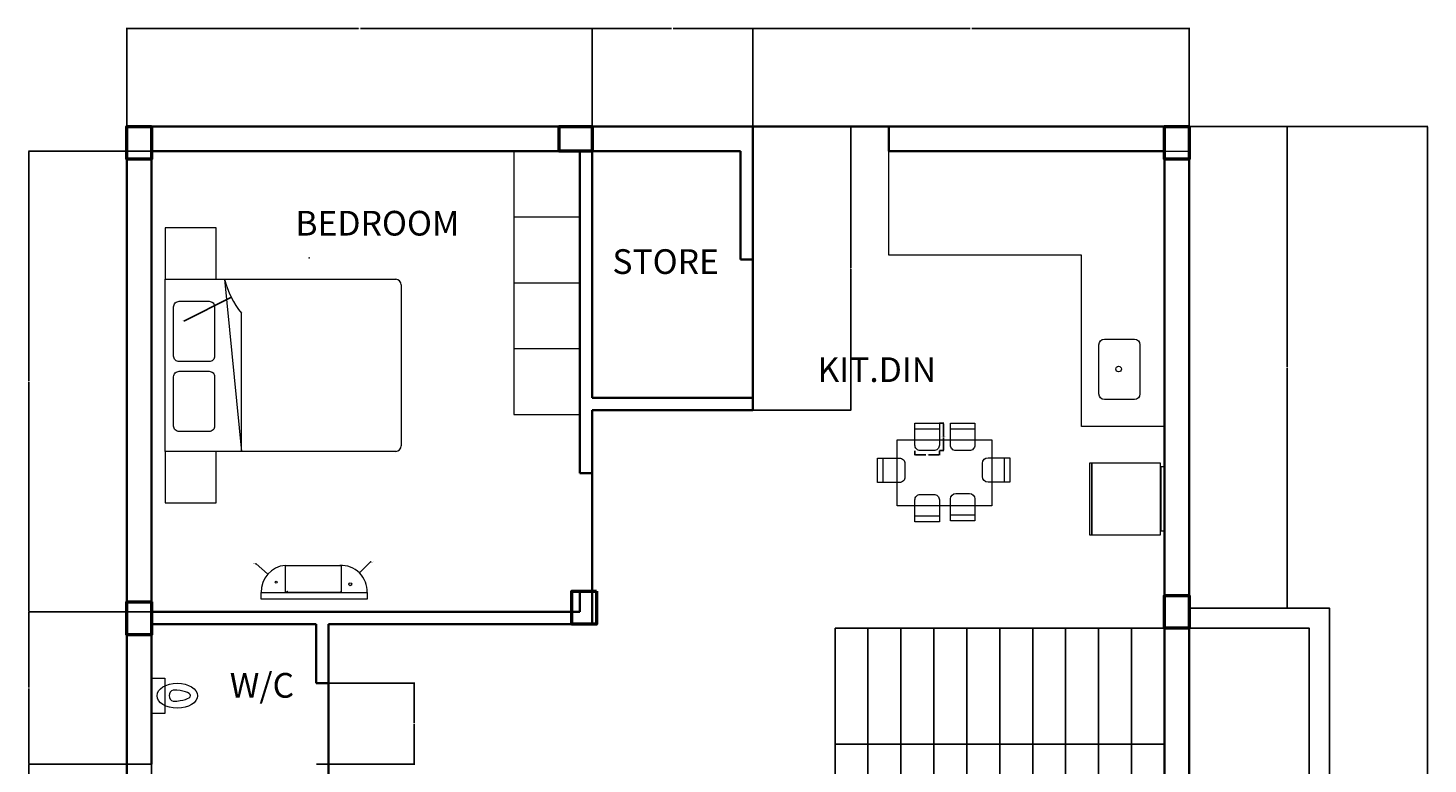
# Model space of a CAD drawing. Units: inches. Extents: x 1748 to 3019, y 1454 to 2188.
# Tile 2 of 4: x 1748 to 2258, y 1919 to 2188. Entities that reach past the tile are written whole.
import ezdxf

# ---------------------------------------------------------------- set-up
doc = ezdxf.new("R2010")
doc.units = ezdxf.units.IN
for name, color, linetype, lineweight in [('A-ANNO-DIMS', 2, 'Continuous', 18), ('A-AREA-IDEN', 134, 'Continuous', 18), ('A-COLS', 120, 'Continuous', 50), ('A-EQPM', 9, 'Continuous', 18), ('A-FLOR-CASE', 9, 'Continuous', 18), ('A-WALL', 7, 'Continuous', 35), ('bathroom', 54, 'Continuous', 18), ('bed', 21, 'Continuous', 18), ('cupboard', 201, 'Continuous', 18), ('dining table', 24, 'Continuous', 18), ('mirror', 149, 'Continuous', 18), ('stairs', 64, 'Continuous', 25), ('washbasin', 106, 'Continuous', 18)]:
    doc.layers.add(name, color=color, linetype=linetype, lineweight=lineweight)
doc.styles.get("Standard").update_dxf_attribs({"font": 'arial.ttf'})
doc.dimstyles.get("Standard").update_dxf_attribs({"dimtxt": 0.18, "dimasz": 0.18, "dimexe": 0.18, "dimexo": 0.0625, "dimgap": 0.09, "dimtad": 0, "dimtih": 1, "dimtoh": 1, "dimdec": 4, "dimzin": 0, "dimdsep": 46, "dimtxsty": 'Standard', "dimcen": 0.09, "dimadec": 0, "dimazin": 0, "dimtfac": 1, "dimtdec": 4, "dimtofl": 0, "dimtmove": 0, "dimatfit": 3, "dimfxl": 1, "dimtolj": 1, "dimtzin": 0, "dimarcsym": 0})

# ---------------------------------------------------------------- blocks, each defined once
blk = doc.blocks.new('BED-DOUBLE-NIGHTSTANDS')
for p, q in [((0, 81.51), (83.98, 81.51)), ((0, 18.79), (0, 81.51)), ((21.61, 81.51), (27.83, 18.79)), ((85.98, 79.51), (85.98, 20.79)), ((27.83, 18.79), (27.83, 69.19)), ((83.98, 18.79), (0, 18.79))]:
    blk.add_line(p, q)
for points in [[(0, 81.51), (18.52, 81.51), (18.52, 100.3), (0, 100.3)], [(0, 0), (18.52, 0), (18.52, 18.79), (0, 18.79)]]:
    blk.add_lwpolyline(points, close=True)
for points in [[(5.06, 73.49), (16.01, 73.49, -0.414214), (18.01, 71.49), (18.01, 53.51, -0.414214), (16.01, 51.51), (5.06, 51.51, -0.414214), (3.06, 53.51), (3.06, 71.49, -0.414214)], [(5.06, 47.99), (16.01, 47.99, -0.414214), (18.01, 45.99), (18.01, 28.02, -0.414214), (16.01, 26.02), (5.06, 26.02, -0.414214), (3.06, 28.02), (3.06, 45.99, -0.414214)]]:
    blk.add_lwpolyline(points, format="xyb", close=True)
for centre, radius, start, end in [((52.42, 89.31), 31.78, 194.1991, 219.2902), ((83.98, 79.51), 2, 0, 90), ((83.98, 79.51), 2, 0, 90), ((83.98, 20.79), 2, 270, 0)]:
    blk.add_arc(centre, radius, start, end)
blk = doc.blocks.new('WARDROBE-4-BAY')
for p, q in [((24, 96), (0, 96)), ((0, 96), (0, 0)), ((24, 0), (24, 96)), ((0, 72), (24, 72)), ((0, 48), (24, 48)), ((0, 24), (24, 24)), ((0, 0), (24, 0))]:
    blk.add_line(p, q)
blk = doc.blocks.new('WC-CLOSE-COUPLED')
blk.add_lwpolyline([(0, 12.82), (4.89, 12.82), (4.89, 0), (0, 0)], close=True)
blk.add_arc((8.58, 6.47), 2.15, 108.3808, 251.6192)
blk.add_ellipse((9.39, 6.41), major_axis=(7.38, 0), ratio=0.615385)
blk.add_ellipse((7.39, 6.47), major_axis=(6.81, 0), ratio=0.3, start_param=4.786849, end_param=7.779521)
blk = doc.blocks.new('DINING-CHAIR')
blk.add_line((0, 7.93), (8.91, 7.93))
blk.add_lwpolyline([(0, 9.99), (8.91, 9.99), (8.91, 2, -0.414214), (6.91, 0), (2, 0, -0.414214), (0, 2)], format="xyb", close=True)
blk = doc.blocks.new('STAIR-FLIGHT-LANDING')
for p, q in [((0, 91.88), (129, 91.88)), ((0, 91.88), (0, 7.38)), ((12, 91.88), (12, 7.38)), ((24, 91.88), (24, 7.38)), ((36, 91.88), (36, 7.38)), ((48, 91.88), (48, 7.38)), ((60, 91.88), (60, 7.38)), ((72, 91.88), (72, 7.38)), ((84, 91.88), (84, 7.38)), ((96, 91.88), (96, 7.38)), ((108, 91.88), (108, 7.38)), ((120, 91.88), (120, 7.38)), ((0, 49.63), (120, 49.63)), ((129, 7.38), (0, 7.38))]:
    blk.add_line(p, q)
blk.add_lwpolyline([(129, 99.26), (180.11, 99.26), (180.11, 0), (129, 0)])
blk.add_lwpolyline([(129, 91.88), (172.73, 91.88), (172.73, 7.38), (129, 7.38)], close=True)
blk = doc.blocks.new('COLUMN-9X12')
blk.add_lwpolyline([(9, 12), (9, 0), (0, 0), (0, 12)], close=True)
blk = doc.blocks.new('*D16')
at = {"layer": 'A-ANNO-DIMS', "color": 0, "lineweight": -2, "transparency": 16777216}
for p, q in [((2079.85, 2043.72), (2081.46, 2043.72)), ((2081.28, 2043.54), (2081.28, 2038.9)), ((2081.28, 2033.9), (2081.28, 2038.54)), ((2079.85, 2033.72), (2081.46, 2033.72))]:
    blk.add_line(p, q, dxfattribs=at)
at = {"layer": 'A-ANNO-DIMS', "color": 0, "transparency": 16777216}
for points in [[(2081.25, 2043.54), (2081.31, 2043.54), (2081.28, 2043.72)], [(2081.25, 2033.9), (2081.31, 2033.9), (2081.28, 2033.72)]]:
    blk.add_solid(points, dxfattribs=at)
at = {"layer": 'Defpoints', "color": 0, "transparency": 16777216}
for p in [(2079.78, 2043.72), (2081.28, 2043.72), (2079.78, 2033.72)]:
    blk.add_point(p, dxfattribs=at)
at = {"layer": 'A-ANNO-DIMS', "color": 0, "transparency": 16777216, "insert": (2081.28, 2038.72), "char_height": 0.18, "attachment_point": 5}
blk.add_mtext('\\A1;CHAIR 10 TYP.', dxfattribs=at)
blk = doc.blocks.new('*D17')
at = {"layer": 'A-ANNO-DIMS', "color": 0, "lineweight": -2, "transparency": 16777216}
for p, q in [((2070.87, 2033.66), (2070.87, 2032.05)), ((2071.05, 2032.23), (2074.87, 2032.23)), ((2079.6, 2032.23), (2075.79, 2032.23)), ((2079.78, 2033.66), (2079.78, 2032.05))]:
    blk.add_line(p, q, dxfattribs=at)
at = {"layer": 'A-ANNO-DIMS', "color": 0, "transparency": 16777216}
for points in [[(2071.05, 2032.26), (2071.05, 2032.2), (2070.87, 2032.23)], [(2079.6, 2032.26), (2079.6, 2032.2), (2079.78, 2032.23)]]:
    blk.add_solid(points, dxfattribs=at)
at = {"layer": 'Defpoints', "color": 0, "transparency": 16777216}
for p in [(2070.87, 2033.72), (2079.78, 2033.72), (2079.78, 2032.23)]:
    blk.add_point(p, dxfattribs=at)
at = {"layer": 'A-ANNO-DIMS', "color": 0, "transparency": 16777216, "insert": (2075.33, 2032.23), "char_height": 0.18, "attachment_point": 5}
blk.add_mtext('\\A1;9 TYP.', dxfattribs=at)
blk = doc.blocks.new('*D23')
at = {"layer": 'A-ANNO-DIMS', "color": 0, "lineweight": -2, "transparency": 16777216}
for p, q in [((2170.84, 2151.94), (2257.77, 2151.94)), ((2257.59, 2151.76), (2257.59, 1870.12)), ((2257.59, 1588.12), (2257.59, 1869.76)), ((2125.84, 1587.94), (2257.77, 1587.94))]:
    blk.add_line(p, q, dxfattribs=at)
at = {"layer": 'A-ANNO-DIMS', "color": 0, "transparency": 16777216}
for points in [[(2257.56, 2151.76), (2257.62, 2151.76), (2257.59, 2151.94)], [(2257.56, 1588.12), (2257.62, 1588.12), (2257.59, 1587.94)]]:
    blk.add_solid(points, dxfattribs=at)
at = {"layer": 'Defpoints', "color": 0, "transparency": 16777216}
for p in [(2170.78, 2151.94), (2257.59, 2151.94), (2125.78, 1587.94)]:
    blk.add_point(p, dxfattribs=at)
at = {"layer": 'A-ANNO-DIMS', "color": 0, "transparency": 16777216, "insert": (2257.59, 1869.94), "char_height": 0.18, "attachment_point": 5}
blk.add_mtext('\\A1;564', dxfattribs=at)
blk = doc.blocks.new('*D24')
at = {"layer": 'A-ANNO-DIMS', "color": 0, "lineweight": -2, "transparency": 16777216}
for p, q in [((1783.78, 2152), (1783.78, 2187.82)), ((1783.96, 2187.64), (1868.15, 2187.64)), ((1953.1, 2187.64), (1868.92, 2187.64)), ((1953.28, 2152), (1953.28, 2187.82))]:
    blk.add_line(p, q, dxfattribs=at)
at = {"layer": 'A-ANNO-DIMS', "color": 0, "transparency": 16777216}
for points in [[(1783.96, 2187.67), (1783.96, 2187.61), (1783.78, 2187.64)], [(1953.1, 2187.67), (1953.1, 2187.61), (1953.28, 2187.64)]]:
    blk.add_solid(points, dxfattribs=at)
at = {"layer": 'Defpoints', "color": 0, "transparency": 16777216}
for p in [(1953.28, 2187.64), (1783.78, 2151.94), (1953.28, 2151.94)]:
    blk.add_point(p, dxfattribs=at)
at = {"layer": 'A-ANNO-DIMS', "color": 0, "transparency": 16777216, "insert": (1868.53, 2187.64), "char_height": 0.18, "attachment_point": 5}
blk.add_mtext('\\A1;169.5', dxfattribs=at)
blk = doc.blocks.new('*D25')
at = {"layer": 'A-ANNO-DIMS', "color": 0, "lineweight": -2, "transparency": 16777216}
for p, q in [((1953.28, 2152), (1953.28, 2187.82)), ((1953.46, 2187.64), (1982.21, 2187.64)), ((2011.6, 2187.64), (1982.86, 2187.64)), ((2011.78, 2152), (2011.78, 2187.82))]:
    blk.add_line(p, q, dxfattribs=at)
at = {"layer": 'A-ANNO-DIMS', "color": 0, "transparency": 16777216}
for points in [[(1953.46, 2187.67), (1953.46, 2187.61), (1953.28, 2187.64)], [(2011.6, 2187.67), (2011.6, 2187.61), (2011.78, 2187.64)]]:
    blk.add_solid(points, dxfattribs=at)
at = {"layer": 'Defpoints', "color": 0, "transparency": 16777216}
for p in [(2011.78, 2187.64), (1953.28, 2151.94), (2011.78, 2151.94)]:
    blk.add_point(p, dxfattribs=at)
at = {"layer": 'A-ANNO-DIMS', "color": 0, "transparency": 16777216, "insert": (1982.53, 2187.64), "char_height": 0.18, "attachment_point": 5}
blk.add_mtext('\\A1;58.5', dxfattribs=at)
blk = doc.blocks.new('*D26')
at = {"layer": 'A-ANNO-DIMS', "color": 0, "lineweight": -2, "transparency": 16777216}
for p, q in [((2011.78, 2152), (2011.78, 2187.82)), ((2011.96, 2187.64), (2091, 2187.64)), ((2170.6, 2187.64), (2091.56, 2187.64)), ((2170.78, 2152), (2170.78, 2187.82))]:
    blk.add_line(p, q, dxfattribs=at)
at = {"layer": 'A-ANNO-DIMS', "color": 0, "transparency": 16777216}
for points in [[(2011.96, 2187.67), (2011.96, 2187.61), (2011.78, 2187.64)], [(2170.6, 2187.67), (2170.6, 2187.61), (2170.78, 2187.64)]]:
    blk.add_solid(points, dxfattribs=at)
at = {"layer": 'Defpoints', "color": 0, "transparency": 16777216}
for p in [(2170.78, 2187.64), (2011.78, 2151.94), (2170.78, 2151.94)]:
    blk.add_point(p, dxfattribs=at)
at = {"layer": 'A-ANNO-DIMS', "color": 0, "transparency": 16777216, "insert": (2091.28, 2187.64), "char_height": 0.18, "attachment_point": 5}
blk.add_mtext('\\A1;159', dxfattribs=at)
blk = doc.blocks.new('*D28')
at = {"layer": 'A-ANNO-DIMS', "color": 0, "lineweight": -2, "transparency": 16777216}
for p, q in [((1792.72, 1919.44), (1747.9, 1919.44)), ((1748.08, 1919.26), (1748.08, 1889.6)), ((1748.08, 1859.57), (1748.08, 1889.23)), ((1792.72, 1859.39), (1747.9, 1859.39))]:
    blk.add_line(p, q, dxfattribs=at)
at = {"layer": 'A-ANNO-DIMS', "color": 0, "transparency": 16777216}
for points in [[(1748.05, 1919.26), (1748.11, 1919.26), (1748.08, 1919.44)], [(1748.05, 1859.57), (1748.11, 1859.57), (1748.08, 1859.39)]]:
    blk.add_solid(points, dxfattribs=at)
at = {"layer": 'Defpoints', "color": 0, "transparency": 16777216}
for p in [(1748.08, 1919.44), (1792.78, 1919.44), (1792.78, 1859.39)]:
    blk.add_point(p, dxfattribs=at)
at = {"layer": 'A-ANNO-DIMS', "color": 0, "transparency": 16777216, "insert": (1748.08, 1889.42), "char_height": 0.18, "attachment_point": 5}
blk.add_mtext('\\A1;60.05', dxfattribs=at)
blk = doc.blocks.new('*D29')
at = {"layer": 'A-ANNO-DIMS', "color": 0, "lineweight": -2, "transparency": 16777216}
for p, q in [((1792.72, 1974.94), (1747.9, 1974.94)), ((1748.08, 1974.76), (1748.08, 1947.37)), ((1748.08, 1919.62), (1748.08, 1947.01)), ((1792.72, 1919.44), (1747.9, 1919.44))]:
    blk.add_line(p, q, dxfattribs=at)
at = {"layer": 'A-ANNO-DIMS', "color": 0, "transparency": 16777216}
for points in [[(1748.05, 1974.76), (1748.11, 1974.76), (1748.08, 1974.94)], [(1748.05, 1919.62), (1748.11, 1919.62), (1748.08, 1919.44)]]:
    blk.add_solid(points, dxfattribs=at)
at = {"layer": 'Defpoints', "color": 0, "transparency": 16777216}
for p in [(1748.08, 1974.94), (1792.78, 1974.94), (1792.78, 1919.44)]:
    blk.add_point(p, dxfattribs=at)
at = {"layer": 'A-ANNO-DIMS', "color": 0, "transparency": 16777216, "insert": (1748.08, 1947.19), "char_height": 0.18, "attachment_point": 5}
blk.add_mtext('\\A1;55.5', dxfattribs=at)
blk = doc.blocks.new('*D30')
at = {"layer": 'A-ANNO-DIMS', "color": 0, "lineweight": -2, "transparency": 16777216}
for p, q in [((1792.72, 2142.94), (1747.9, 2142.94)), ((1748.08, 2142.76), (1748.08, 2059.12)), ((1748.08, 1975.12), (1748.08, 2058.76)), ((1792.72, 1974.94), (1747.9, 1974.94))]:
    blk.add_line(p, q, dxfattribs=at)
at = {"layer": 'A-ANNO-DIMS', "color": 0, "transparency": 16777216}
for points in [[(1748.05, 2142.76), (1748.11, 2142.76), (1748.08, 2142.94)], [(1748.05, 1975.12), (1748.11, 1975.12), (1748.08, 1974.94)]]:
    blk.add_solid(points, dxfattribs=at)
at = {"layer": 'Defpoints', "color": 0, "transparency": 16777216}
for p in [(1748.08, 2142.94), (1792.78, 2142.94), (1792.78, 1974.94)]:
    blk.add_point(p, dxfattribs=at)
at = {"layer": 'A-ANNO-DIMS', "color": 0, "transparency": 16777216, "insert": (1748.08, 2058.94), "char_height": 0.18, "attachment_point": 5}
blk.add_mtext('\\A1;168', dxfattribs=at)
blk = doc.blocks.new('*D31')
at = {"layer": 'A-ANNO-DIMS', "color": 0, "lineweight": -2, "transparency": 16777216}
for p, q in [((1792.78, 1970.38), (1792.78, 1552.06)), ((1857.28, 1970.38), (1857.28, 1552.06)), ((1792.96, 1552.24), (1824.71, 1552.24)), ((1857.1, 1552.24), (1825.36, 1552.24))]:
    blk.add_line(p, q, dxfattribs=at)
at = {"layer": 'A-ANNO-DIMS', "color": 0, "transparency": 16777216}
for points in [[(1792.96, 1552.27), (1792.96, 1552.21), (1792.78, 1552.24)], [(1857.1, 1552.27), (1857.1, 1552.21), (1857.28, 1552.24)]]:
    blk.add_solid(points, dxfattribs=at)
at = {"layer": 'Defpoints', "color": 0, "transparency": 16777216}
for p in [(1792.78, 1970.44), (1857.28, 1970.44), (1857.28, 1552.24)]:
    blk.add_point(p, dxfattribs=at)
at = {"layer": 'A-ANNO-DIMS', "color": 0, "transparency": 16777216, "insert": (1825.03, 1552.24), "char_height": 0.18, "attachment_point": 5}
blk.add_mtext('\\A1;64.5', dxfattribs=at)
blk = doc.blocks.new('*D33')
at = {"layer": 'A-ANNO-DIMS', "color": 0, "lineweight": -2, "transparency": 16777216}
for p, q in [((2011.84, 2151.94), (2047.66, 2151.94)), ((2047.48, 2151.76), (2047.48, 2100.37)), ((2047.48, 2048.62), (2047.48, 2100.01)), ((2011.84, 2048.44), (2047.66, 2048.44))]:
    blk.add_line(p, q, dxfattribs=at)
at = {"layer": 'A-ANNO-DIMS', "color": 0, "transparency": 16777216}
for points in [[(2047.45, 2151.76), (2047.51, 2151.76), (2047.48, 2151.94)], [(2047.45, 2048.62), (2047.51, 2048.62), (2047.48, 2048.44)]]:
    blk.add_solid(points, dxfattribs=at)
at = {"layer": 'Defpoints', "color": 0, "transparency": 16777216}
for p in [(2011.78, 2151.94), (2011.78, 2048.44), (2047.48, 2048.44)]:
    blk.add_point(p, dxfattribs=at)
at = {"layer": 'A-ANNO-DIMS', "color": 0, "transparency": 16777216, "insert": (2047.48, 2100.19), "char_height": 0.18, "attachment_point": 5}
blk.add_mtext('\\A1;103.5', dxfattribs=at)
blk = doc.blocks.new('*D41')
at = {"layer": 'A-ANNO-DIMS', "color": 0, "lineweight": -2, "transparency": 16777216}
for p, q in [((2170.84, 2151.94), (2206.66, 2151.94)), ((2206.48, 2151.76), (2206.48, 2064.31)), ((2206.48, 1976.5), (2206.48, 2063.95)), ((2170.84, 1976.32), (2206.66, 1976.32))]:
    blk.add_line(p, q, dxfattribs=at)
at = {"layer": 'A-ANNO-DIMS', "color": 0, "transparency": 16777216}
for points in [[(2206.45, 2151.76), (2206.51, 2151.76), (2206.48, 2151.94)], [(2206.45, 1976.5), (2206.51, 1976.5), (2206.48, 1976.32)]]:
    blk.add_solid(points, dxfattribs=at)
at = {"layer": 'Defpoints', "color": 0, "transparency": 16777216}
for p in [(2170.78, 2151.94), (2170.78, 1976.32), (2206.48, 1976.32)]:
    blk.add_point(p, dxfattribs=at)
at = {"layer": 'A-ANNO-DIMS', "color": 0, "transparency": 16777216, "insert": (2206.48, 2064.13), "char_height": 0.18, "attachment_point": 5}
blk.add_mtext('\\A1;175.62', dxfattribs=at)
blk = doc.blocks.new('*D43')
at = {"layer": 'A-ANNO-DIMS', "color": 0, "lineweight": -2, "transparency": 16777216}
for p, q in [((1852.84, 1948.95), (1888.66, 1948.95)), ((1888.48, 1948.77), (1888.48, 1934.38)), ((1888.48, 1919.62), (1888.48, 1934.02)), ((1852.84, 1919.44), (1888.66, 1919.44))]:
    blk.add_line(p, q, dxfattribs=at)
at = {"layer": 'A-ANNO-DIMS', "color": 0, "transparency": 16777216}
for points in [[(1888.45, 1948.77), (1888.51, 1948.77), (1888.48, 1948.95)], [(1888.45, 1919.62), (1888.51, 1919.62), (1888.48, 1919.44)]]:
    blk.add_solid(points, dxfattribs=at)
at = {"layer": 'Defpoints', "color": 0, "transparency": 16777216}
for p in [(1852.78, 1948.95), (1852.78, 1919.44), (1888.48, 1919.44)]:
    blk.add_point(p, dxfattribs=at)
at = {"layer": 'A-ANNO-DIMS', "color": 0, "transparency": 16777216, "insert": (1888.48, 1934.2), "char_height": 0.18, "attachment_point": 5}
blk.add_mtext('\\A1;29.515', dxfattribs=at)
blk = doc.blocks.new('*D65')
at = {"layer": 'A-ANNO-DIMS', "color": 0, "lineweight": -2, "transparency": 16777216}
for p, q in [((1850.09, 2103.97), (1850.27, 2103.97)), ((1850.18, 2103.88), (1850.18, 2104.06)), ((1804.78, 2081.09), (1821.65, 2089.59)), ((1804.6, 2081.09), (1804.78, 2081.09))]:
    blk.add_line(p, q, dxfattribs=at)
at = {"layer": 'A-ANNO-DIMS', "color": 0, "transparency": 16777216}
blk.add_solid([(1821.63, 2089.62), (1821.66, 2089.56), (1821.81, 2089.67)], dxfattribs=at)
at = {"layer": 'Defpoints', "color": 0, "transparency": 16777216}
for p in [(1850.18, 2103.97), (1821.81, 2089.67)]:
    blk.add_point(p, dxfattribs=at)
at = {"layer": 'A-ANNO-DIMS', "color": 0, "transparency": 16777216, "insert": (1804.12, 2081.09), "char_height": 0.18, "attachment_point": 5}
blk.add_mtext('\\A1;R31.78', dxfattribs=at)
blk = doc.blocks.new('*D66')
at = {"layer": 'A-ANNO-DIMS', "color": 0, "lineweight": -2, "transparency": 16777216}
for p, q in [((1830.69, 1992.48), (1830.87, 1992.48)), ((1830.87, 1992.48), (1834.99, 1988.82)), ((1842.13, 1982.39), (1842.31, 1982.39)), ((1842.22, 1982.3), (1842.22, 1982.48))]:
    blk.add_line(p, q, dxfattribs=at)
at = {"layer": 'A-ANNO-DIMS', "color": 0, "transparency": 16777216}
blk.add_solid([(1835.01, 1988.84), (1834.97, 1988.8), (1835.13, 1988.7)], dxfattribs=at)
at = {"layer": 'Defpoints', "color": 0, "transparency": 16777216}
for p in [(1835.13, 1988.7), (1842.22, 1982.39)]:
    blk.add_point(p, dxfattribs=at)
at = {"layer": 'A-ANNO-DIMS', "color": 0, "transparency": 16777216, "insert": (1830.21, 1992.48), "char_height": 0.18, "attachment_point": 5}
blk.add_mtext('\\A1;R9.493', dxfattribs=at)
blk = doc.blocks.new('*D67')
at = {"layer": 'A-ANNO-DIMS', "color": 0, "lineweight": -2, "transparency": 16777216}
for p, q in [((1872.56, 1993.12), (1868.67, 1989.22)), ((1872.74, 1993.12), (1872.56, 1993.12)), ((1861.76, 1982.39), (1861.94, 1982.39)), ((1861.85, 1982.3), (1861.85, 1982.48))]:
    blk.add_line(p, q, dxfattribs=at)
at = {"layer": 'A-ANNO-DIMS', "color": 0, "transparency": 16777216}
blk.add_solid([(1868.65, 1989.24), (1868.69, 1989.2), (1868.54, 1989.09)], dxfattribs=at)
at = {"layer": 'Defpoints', "color": 0, "transparency": 16777216}
for p in [(1868.54, 1989.09), (1861.85, 1982.39)]:
    blk.add_point(p, dxfattribs=at)
at = {"layer": 'A-ANNO-DIMS', "color": 0, "transparency": 16777216, "insert": (1873.22, 1993.12), "char_height": 0.18, "attachment_point": 5}
blk.add_mtext('\\A1;R9.474', dxfattribs=at)

msp = doc.modelspace()

# ---------------------------------------------------------------- linework, layer by layer
at = {"layer": 'A-EQPM'}
for points in [[(2135.3461, 2029.0905), (2134.5193, 2029.0905), (2134.5193, 2002.968), (2135.3461, 2002.968)], [(2160.3093, 2029.0905), (2135.3461, 2029.0905), (2135.3461, 2002.969), (2160.3093, 2002.969)], [(2135.3461, 2029.0905), (2135.3461, 2029.0905), (2135.3461, 2002.969), (2135.3461, 2002.969)], [(2161.7824, 2027.8069), (2160.4246, 2027.8069), (2160.4246, 2004.4644), (2161.7824, 2004.4644)], [(2161.7824, 2027.8069), (2161.7824, 2027.8069), (2161.7824, 2004.8656), (2161.7824, 2004.8656)]]:
    msp.add_lwpolyline(points, close=True, dxfattribs=at)
at = {"layer": 'A-FLOR-CASE'}
for points in [[(2131.5284, 2104.9964), (2061.3307, 2104.9964), (2061.3307, 2142.94), (2170.7824, 2142.94)], [(2131.5284, 2142.94), (2161.7824, 2142.94)], [(2161.7824, 2042.4759), (2131.5284, 2042.4759), (2131.5284, 2104.9964)]]:
    msp.add_lwpolyline(points, dxfattribs=at)
at = {"layer": 'A-WALL'}
for p, q in [((2011.7824, 2048.44), (2011.7824, 2151.94)), ((2061.3307, 2142.94), (2061.3307, 2151.94)), ((1792.7824, 2142.94), (1948.7824, 2142.94)), ((1792.7824, 1974.94), (1792.7824, 2142.94)), ((1948.7824, 2025.5144), (1948.7824, 2142.94)), ((1953.2824, 2052.94), (1953.2824, 2142.94)), ((1953.2824, 2142.94), (2007.2824, 2142.94)), ((2007.2824, 2103.3583), (2007.2824, 2142.94)), ((2061.3307, 2142.94), (2161.7824, 2142.94)), ((2161.7824, 2142.94), (2161.7824, 1709.44)), ((2007.2824, 2103.3583), (2011.7824, 2103.3583)), ((1953.2824, 2052.94), (2011.7824, 2052.94)), ((1953.2824, 2048.44), (2011.7824, 2048.44)), ((1953.2824, 1970.44), (1953.2824, 2048.44)), ((1948.7824, 2025.5144), (1953.2824, 2025.5144)), ((1953.2824, 2026.1397), (1953.2824, 2026.1397)), ((1948.7824, 1974.94), (1948.7824, 1982.44)), ((1792.7824, 1974.94), (1948.7824, 1974.94)), ((1792.7824, 1970.44), (1852.7824, 1970.44)), ((1792.7824, 1919.44), (1792.7824, 1970.44)), ((1852.7824, 1948.9549), (1852.7824, 1970.44)), ((1857.2824, 1914.94), (1857.2824, 1970.44)), ((1857.2824, 1970.44), (1953.2824, 1970.44)), ((1852.7824, 1948.9549), (1857.2824, 1948.9549))]:
    msp.add_line(p, q, dxfattribs=at)
msp.add_lwpolyline([(2125.7824, 1587.94), (1783.7824, 1587.94), (1783.7824, 2151.94), (2170.7824, 2151.94), (2170.7824, 1709.44)], dxfattribs=at)
at = {"layer": 'dining table'}
for p, q in [((2103.4314, 2031.1443), (2103.4314, 2022.2317)), ((2092.7252, 2010.1641), (2083.8126, 2010.1641))]:
    msp.add_line(p, q, dxfattribs=at)
msp.add_lwpolyline([(2064.3974, 2037.6338), (2098.8785, 2037.6338), (2098.8785, 2013.6044), (2064.3974, 2013.6044)], close=True, dxfattribs=at)
for points in [[(2105.4972, 2031.1443), (2105.4972, 2022.2317), (2097.5033, 2022.2317, -0.41421356), (2095.5033, 2024.2317), (2095.5033, 2029.1443, -0.41421356), (2097.5033, 2031.1443)], [(2092.7252, 2008.0983), (2083.8126, 2008.0983), (2083.8126, 2016.0922, -0.41421356), (2085.8126, 2018.0922), (2090.7252, 2018.0922, -0.41421356), (2092.7252, 2016.0922)]]:
    msp.add_lwpolyline(points, format="xyb", close=True, dxfattribs=at)
at = {"layer": 'mirror'}
for points in [[(1841.5637, 1991.8643), (1861.842, 1991.8643), (1861.842, 1981.9368), (1841.5637, 1981.9368)], [(1832.7431, 1981.9368), (1871.3117, 1981.9368), (1871.3117, 1979.5641), (1832.7431, 1979.5641)]]:
    msp.add_lwpolyline(points, close=True, dxfattribs=at)
for centre, radius in [((1838.191, 1985.7496), 0.3775), ((1865.1857, 1984.9949), 0.5276)]:
    msp.add_circle(centre, radius, dxfattribs=at)
for centre, radius, start, end in [((1842.2248, 1982.3946), 9.4927, 93.993397, 182.764418), ((1861.8489, 1982.3909), 9.4738, 357.252549, 92.811242)]:
    msp.add_arc(centre, radius, start, end, dxfattribs=at)
at = {"layer": 'washbasin'}
msp.add_lwpolyline([(2139.9102, 2074.3401), (2150.8631, 2074.3401, -0.41421356), (2152.8631, 2072.3401), (2152.8631, 2054.3628, -0.41421356), (2150.8631, 2052.3628), (2139.9102, 2052.3628, -0.41421356), (2137.9102, 2054.3628), (2137.9102, 2072.3401, -0.41421356)], format="xyb", close=True, dxfattribs=at)
msp.add_circle((2145.0826, 2063.4508), 1.0067, dxfattribs=at)

# ---------------------------------------------------------------- block references
at = {"layer": 'A-COLS'}
for p in [(1783.782, 2139.94), (2161.782, 2139.94), (1945.8338, 1970.44), (2161.782, 1968.94), (1783.782, 1966.5724)]:
    msp.add_blockref('COLUMN-9X12', p, dxfattribs=at)
at = {"layer": 'A-COLS', "rotation": 269.9999999999997}
msp.add_blockref('COLUMN-9X12', (1941.2824, 2151.9404), dxfattribs=at)
at = {"layer": 'bathroom'}
msp.add_blockref('WC-CLOSE-COUPLED', (1792.782, 1937.912), dxfattribs=at)
at = {"layer": 'bed'}
msp.add_blockref('BED-DOUBLE-NIGHTSTANDS', (1797.763, 2014.663), dxfattribs=at)
at = {"layer": 'cupboard'}
msp.add_blockref('WARDROBE-4-BAY', (1924.782, 2046.94), dxfattribs=at)
at = {"layer": 'dining table'}
for p in [(2070.871, 2033.725), (2083.8127, 2033.725)]:
    msp.add_blockref('DINING-CHAIR', p, dxfattribs=at)
for p, rotation in [((2067.259, 2022.0607), 89.99999999999811), ((2079.7835, 2017.75), 180)]:
    msp.add_blockref('DINING-CHAIR', p, dxfattribs=dict(at, rotation=rotation))
at = {"layer": 'stairs'}
msp.add_blockref('STAIR-FLIGHT-LANDING', (2041.782, 1877.058), dxfattribs=at)

# ---------------------------------------------------------------- texts
at = {"layer": 'A-AREA-IDEN', "char_height": 9, "attachment_point": 1}
for s, width, insert in [('BEDROOM', 14.161869, (1845.1787, 2121.131)), ('STORE', 23.468243, (1960.6665, 2107.1397)), ('KIT.DIN', 51.387342, (2035.3875, 2067.7329)), ('W/C', 8.853532, (1821.2747, 1952.6253))]:
    msp.add_mtext_dynamic_manual_height_columns(s, width=width, gutter_width=12.5, heights=[0], dxfattribs=dict(at, insert=insert))

# ---------------------------------------------------------------- dimensions: what is measured, and where the dimension line sits
at = {"layer": 'A-ANNO-DIMS'}
for base, p1, p2, override, picture, middle in [((1953.2824, 2187.64), (1783.7824, 2151.94), (1953.2824, 2151.94), {"dimdec": 1, "dimlfac": 1, "dimrnd": 0, "dimzin": 0, "dimdsep": 46, "dimlunit": 2}, '*D24', (1868.5324, 2187.64)), ((2011.7824, 2187.64), (1953.2824, 2151.94), (2011.7824, 2151.94), {"dimdec": 1, "dimlfac": 1, "dimrnd": 0, "dimzin": 0, "dimdsep": 46, "dimlunit": 2}, '*D25', (1982.5324, 2187.64)), ((2170.7824, 2187.64), (2011.7824, 2151.94), (2170.7824, 2151.94), {"dimdec": 0, "dimlfac": 1, "dimrnd": 0, "dimzin": 0, "dimdsep": 46, "dimlunit": 2}, '*D26', (2091.2824, 2187.64)), ((1857.2824, 1552.24), (1792.7824, 1970.44), (1857.2824, 1970.44), {"dimdec": 1, "dimlfac": 1, "dimrnd": 0, "dimzin": 0, "dimdsep": 46, "dimlunit": 2}, '*D31', (1825.0324, 1552.24))]:
    dim = msp.add_linear_dim(base=base, p1=p1, p2=p2, dimstyle='Standard', override=override, dxfattribs=at)
    dim.commit()
    dim.dimension.update_dxf_attribs({"geometry": picture, "text_midpoint": middle})
for base, p1, p2, angle, override, picture, middle in [((2047.4824, 2048.44), (2011.7824, 2151.94), (2011.7824, 2048.44), 270, {"dimdec": 1, "dimlfac": 1, "dimrnd": 0, "dimzin": 0, "dimdsep": 46, "dimlunit": 2}, '*D33', (2047.4824, 2100.19)), ((2257.5899, 2151.94), (2125.7824, 1587.94), (2170.7824, 2151.94), 90, {"dimdec": 0, "dimlfac": 1, "dimrnd": 0, "dimzin": 0, "dimdsep": 46, "dimlunit": 2}, '*D23', (2257.5899, 1869.94)), ((2206.4824, 1976.3216), (2170.7824, 2151.94), (2170.7824, 1976.3216), 270, {"dimdec": 2, "dimlfac": 1, "dimrnd": 0, "dimzin": 0, "dimdsep": 46, "dimlunit": 2}, '*D41', (2206.4824, 2064.1308)), ((1748.0824, 2142.94), (1792.7824, 1974.94), (1792.7824, 2142.94), 90, {"dimdec": 0, "dimlfac": 1, "dimrnd": 0, "dimzin": 0, "dimdsep": 46, "dimlunit": 2}, '*D30', (1748.0824, 2058.94)), ((1748.0824, 1974.94), (1792.7824, 1919.44), (1792.7824, 1974.94), 90, {"dimdec": 1, "dimlfac": 1, "dimrnd": 0, "dimzin": 0, "dimdsep": 46, "dimlunit": 2}, '*D29', (1748.0824, 1947.19)), ((1888.4824, 1919.44), (1852.7824, 1948.9549), (1852.7824, 1919.44), 270, {"dimdec": 3, "dimlfac": 1, "dimrnd": 0, "dimzin": 0, "dimdsep": 46, "dimlunit": 2}, '*D43', (1888.4824, 1934.1975)), ((1748.0824, 1919.44), (1792.7824, 1859.3932), (1792.7824, 1919.44), 90, {"dimdec": 2, "dimlfac": 1, "dimrnd": 0, "dimzin": 0, "dimdsep": 46, "dimlunit": 2}, '*D28', (1748.0824, 1889.4166))]:
    dim = msp.add_linear_dim(base=base, p1=p1, p2=p2, angle=angle, dimstyle='Standard', override=override, dxfattribs=at)
    dim.commit()
    dim.dimension.update_dxf_attribs({"geometry": picture, "text_midpoint": middle})
for center, mpoint, override, picture, middle in [((1850.1835, 2103.9716), (1821.8061, 2089.671), {"dimdec": 2, "dimlfac": 1, "dimrnd": 0, "dimzin": 0, "dimdsep": 46, "dimlunit": 2}, '*D65', (1804.1196, 2081.0907)), ((1842.2248, 1982.3946), (1835.1289, 1988.7001), {"dimdec": 3, "dimlfac": 1, "dimrnd": 0, "dimzin": 0, "dimdsep": 46, "dimlunit": 2}, '*D66', (1830.2114, 1992.4834)), ((1861.8489, 1982.3909), (1868.5438, 1989.0938), {"dimdec": 3, "dimlfac": 1, "dimrnd": 0, "dimzin": 0, "dimdsep": 46, "dimlunit": 2}, '*D67', (1873.2203, 1993.1156))]:
    dim = msp.add_radius_dim(center=center, mpoint=mpoint, dimstyle='Standard', override=override, dxfattribs=at)
    dim.commit()
    dim.dimension.update_dxf_attribs({"geometry": picture, "text_midpoint": middle, "dimtype": 164})
dim = msp.add_linear_dim(base=(2081.2827, 2043.7188), p1=(2079.7836, 2033.7248), p2=(2079.7836, 2043.7188), angle=90, text='CHAIR <> TYP.', dimstyle='Standard', override={"dimdec": 0, "dimlfac": 1, "dimrnd": 0, "dimzin": 0, "dimdsep": 46, "dimlunit": 2}, dxfattribs=at)
dim.commit()
dim.dimension.update_dxf_attribs({"geometry": '*D16', "text_midpoint": (2081.2827, 2038.7218)})
dim = msp.add_linear_dim(base=(2079.7836, 2032.2257), p1=(2070.871, 2033.7248), p2=(2079.7836, 2033.7248), text='<> TYP.', dimstyle='Standard', override={"dimdec": 0, "dimlfac": 1, "dimrnd": 0, "dimzin": 0, "dimdsep": 46, "dimlunit": 2}, dxfattribs=at)
dim.commit()
dim.dimension.update_dxf_attribs({"geometry": '*D17', "text_midpoint": (2075.3273, 2032.2257)})

doc.saveas('drawing.dxf')
